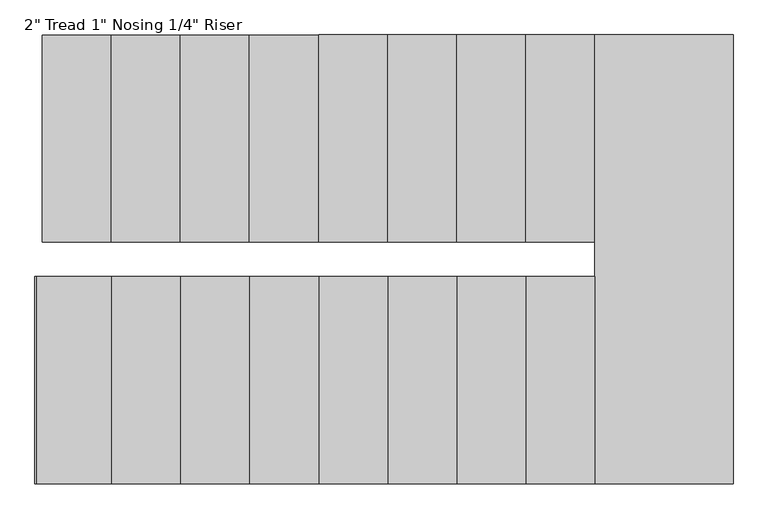
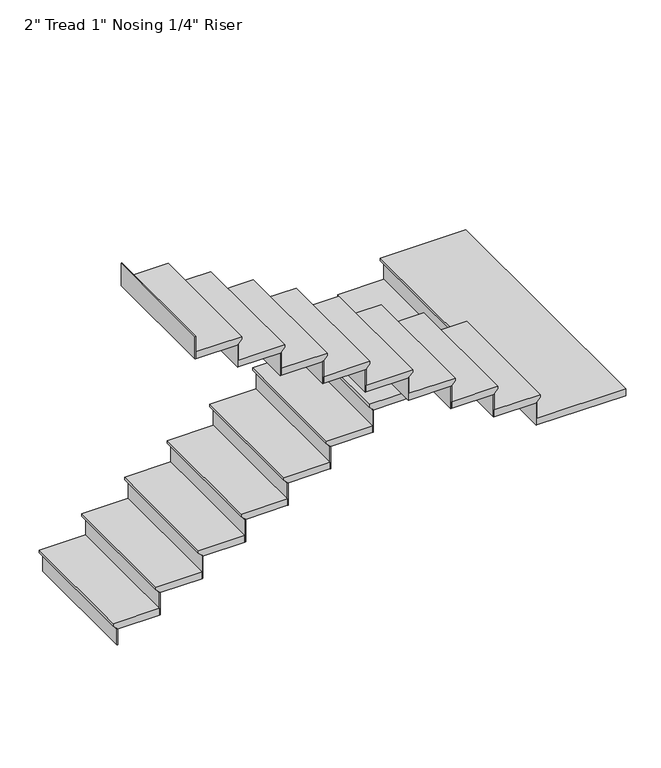
"""IFC4 building model written with IfcOpenShell, lengths in millimetres: stair flight geometry."""

from ifc_helpers import new_model, si_unit, origin, place, context, project, spatial, faceted_brep, source, transform, mapped, element, save


def stair_flight_ef7e9c63(model_context):
    return source(origin(), model_context, "Body", "Brep", [
        faceted_brep([(4699.0, 4356.1, 6246.2833333), (4699.0, 4356.1, 6265.3333333), (4699.0, 5270.5, 6265.3333333), (4699.0, 5270.5, 6246.2833333), (4724.4, 4356.1, 6220.8833333), (4724.4, 5270.5, 6220.8833333), (5029.2, 4356.1, 6265.3333333), (5029.2, 5270.5, 6265.3333333), (4724.4, 5270.5, 6214.5333333), (5029.2, 5270.5, 6214.5333333), (5029.2, 4356.1, 6214.5333333), (4724.4, 4356.1, 6214.5333333)], [[[0, 1, 2, 3]], [[4, 0, 3, 5]], [[2, 1, 6, 7]], [[8, 9, 10, 11]], [[2, 7, 9, 8, 5, 3]], [[8, 11, 4, 5]], [[6, 1, 0, 4, 11, 10]], [[7, 6, 10, 9]]]),
        faceted_brep([(4724.4, 4356.1, 6214.5333333), (4724.4, 4356.1, 6096.0), (4730.75, 4356.1, 6096.0), (4730.75, 4356.1, 6214.5333333), (4724.4, 5270.5, 6214.5333333), (4730.75, 5270.5, 6214.5333333), (4730.75, 5270.5, 6096.0), (4724.4, 5270.5, 6096.0)], [[[0, 1, 2, 3]], [[4, 5, 6, 7]], [[1, 0, 4, 7]], [[2, 1, 7, 6]], [[3, 2, 6, 5]], [[0, 3, 5, 4]]]),
        faceted_brep([(5029.2, 4356.1, 6383.8666667), (5029.2, 4356.1, 6214.5333333), (5035.55, 4356.1, 6214.5333333), (5035.55, 4356.1, 6383.8666667), (5029.2, 5270.5, 6383.8666667), (5035.55, 5270.5, 6383.8666667), (5035.55, 5270.5, 6214.5333333), (5029.2, 5270.5, 6214.5333333)], [[[0, 1, 2, 3]], [[4, 5, 6, 7]], [[1, 0, 4, 7]], [[2, 1, 7, 6]], [[3, 2, 6, 5]], [[0, 3, 5, 4]]]),
        faceted_brep([(5003.8, 5270.5, 6434.6666667), (5003.8, 4356.1, 6434.6666667), (5334.0, 4356.1, 6434.6666667), (5334.0, 5270.5, 6434.6666667), (5029.2, 5270.5, 6383.8666667), (5334.0, 5270.5, 6383.8666667), (5334.0, 4356.1, 6383.8666667), (5029.2, 4356.1, 6383.8666667), (5029.2, 5270.5, 6390.2166667), (5003.8, 5270.5, 6415.6166667), (5029.2, 4356.1, 6390.2166667), (5003.8, 4356.1, 6415.6166667)], [[[0, 1, 2, 3]], [[4, 5, 6, 7]], [[0, 3, 5, 4, 8, 9]], [[4, 7, 10, 8]], [[2, 1, 11, 10, 7, 6]], [[3, 2, 6, 5]], [[11, 1, 0, 9]], [[10, 11, 9, 8]]]),
        faceted_brep([(5334.0, 4356.1, 6553.2), (5334.0, 4356.1, 6383.8666667), (5340.35, 4356.1, 6383.8666667), (5340.35, 4356.1, 6553.2), (5334.0, 5270.5, 6553.2), (5340.35, 5270.5, 6553.2), (5340.35, 5270.5, 6383.8666667), (5334.0, 5270.5, 6383.8666667)], [[[0, 1, 2, 3]], [[4, 5, 6, 7]], [[1, 0, 4, 7]], [[2, 1, 7, 6]], [[3, 2, 6, 5]], [[0, 3, 5, 4]]]),
        faceted_brep([(5308.6, 5270.5, 6604.0), (5308.6, 4356.1, 6604.0), (5638.8, 4356.1, 6604.0), (5638.8, 5270.5, 6604.0), (5334.0, 5270.5, 6553.2), (5638.8, 5270.5, 6553.2), (5638.8, 4356.1, 6553.2), (5334.0, 4356.1, 6553.2), (5334.0, 5270.5, 6559.55), (5308.6, 5270.5, 6584.95), (5334.0, 4356.1, 6559.55), (5308.6, 4356.1, 6584.95)], [[[0, 1, 2, 3]], [[4, 5, 6, 7]], [[0, 3, 5, 4, 8, 9]], [[4, 7, 10, 8]], [[2, 1, 11, 10, 7, 6]], [[3, 2, 6, 5]], [[11, 1, 0, 9]], [[10, 11, 9, 8]]]),
        faceted_brep([(5638.8, 4356.1, 6722.5333333), (5638.8, 4356.1, 6553.2), (5645.15, 4356.1, 6553.2), (5645.15, 4356.1, 6722.5333333), (5638.8, 5270.5, 6722.5333333), (5645.15, 5270.5, 6722.5333333), (5645.15, 5270.5, 6553.2), (5638.8, 5270.5, 6553.2)], [[[0, 1, 2, 3]], [[4, 5, 6, 7]], [[1, 0, 4, 7]], [[2, 1, 7, 6]], [[3, 2, 6, 5]], [[0, 3, 5, 4]]]),
        faceted_brep([(5613.4, 5270.5, 6773.3333333), (5613.4, 4356.1, 6773.3333333), (5943.6, 4356.1, 6773.3333333), (5943.6, 5270.5, 6773.3333333), (5638.8, 5270.5, 6722.5333333), (5943.6, 5270.5, 6722.5333333), (5943.6, 4356.1, 6722.5333333), (5638.8, 4356.1, 6722.5333333), (5638.8, 5270.5, 6728.8833333), (5613.4, 5270.5, 6754.2833333), (5638.8, 4356.1, 6728.8833333), (5613.4, 4356.1, 6754.2833333)], [[[0, 1, 2, 3]], [[4, 5, 6, 7]], [[0, 3, 5, 4, 8, 9]], [[4, 7, 10, 8]], [[2, 1, 11, 10, 7, 6]], [[3, 2, 6, 5]], [[11, 1, 0, 9]], [[10, 11, 9, 8]]]),
        faceted_brep([(5943.6, 4356.1, 6891.8666667), (5943.6, 4356.1, 6722.5333333), (5949.95, 4356.1, 6722.5333333), (5949.95, 4356.1, 6891.8666667), (5943.6, 5270.5, 6891.8666667), (5949.95, 5270.5, 6891.8666667), (5949.95, 5270.5, 6722.5333333), (5943.6, 5270.5, 6722.5333333)], [[[0, 1, 2, 3]], [[4, 5, 6, 7]], [[1, 0, 4, 7]], [[2, 1, 7, 6]], [[3, 2, 6, 5]], [[0, 3, 5, 4]]]),
        faceted_brep([(5918.2, 5270.5, 6942.6666667), (5918.2, 4356.1, 6942.6666667), (6248.4, 4356.1, 6942.6666667), (6248.4, 5270.5, 6942.6666667), (5943.6, 5270.5, 6891.8666667), (6248.4, 5270.5, 6891.8666667), (6248.4, 4356.1, 6891.8666667), (5943.6, 4356.1, 6891.8666667), (5943.6, 5270.5, 6898.2166667), (5918.2, 5270.5, 6923.6166667), (5943.6, 4356.1, 6898.2166667), (5918.2, 4356.1, 6923.6166667)], [[[0, 1, 2, 3]], [[4, 5, 6, 7]], [[0, 3, 5, 4, 8, 9]], [[4, 7, 10, 8]], [[2, 1, 11, 10, 7, 6]], [[3, 2, 6, 5]], [[11, 1, 0, 9]], [[10, 11, 9, 8]]]),
        faceted_brep([(6248.4, 4356.1, 7061.2), (6248.4, 4356.1, 6891.8666667), (6254.75, 4356.1, 6891.8666667), (6254.75, 4356.1, 7061.2), (6248.4, 5270.5, 7061.2), (6254.75, 5270.5, 7061.2), (6254.75, 5270.5, 6891.8666667), (6248.4, 5270.5, 6891.8666667)], [[[0, 1, 2, 3]], [[4, 5, 6, 7]], [[1, 0, 4, 7]], [[2, 1, 7, 6]], [[3, 2, 6, 5]], [[0, 3, 5, 4]]]),
        faceted_brep([(6223.0, 5270.5, 7112.0), (6223.0, 4356.1, 7112.0), (6553.2, 4356.1, 7112.0), (6553.2, 5270.5, 7112.0), (6248.4, 5270.5, 7061.2), (6553.2, 5270.5, 7061.2), (6553.2, 4356.1, 7061.2), (6248.4, 4356.1, 7061.2), (6248.4, 5270.5, 7067.55), (6223.0, 5270.5, 7092.95), (6248.4, 4356.1, 7067.55), (6223.0, 4356.1, 7092.95)], [[[0, 1, 2, 3]], [[4, 5, 6, 7]], [[0, 3, 5, 4, 8, 9]], [[4, 7, 10, 8]], [[2, 1, 11, 10, 7, 6]], [[3, 2, 6, 5]], [[11, 1, 0, 9]], [[10, 11, 9, 8]]]),
        faceted_brep([(6553.2, 4356.1, 7230.5333333), (6553.2, 4356.1, 7061.2), (6559.55, 4356.1, 7061.2), (6559.55, 4356.1, 7230.5333333), (6553.2, 5270.5, 7230.5333333), (6559.55, 5270.5, 7230.5333333), (6559.55, 5270.5, 7061.2), (6553.2, 5270.5, 7061.2)], [[[0, 1, 2, 3]], [[4, 5, 6, 7]], [[1, 0, 4, 7]], [[2, 1, 7, 6]], [[3, 2, 6, 5]], [[0, 3, 5, 4]]]),
        faceted_brep([(6527.8, 5270.5, 7281.3333333), (6527.8, 4356.1, 7281.3333333), (6858.0, 4356.1, 7281.3333333), (6858.0, 5270.5, 7281.3333333), (6553.2, 5270.5, 7230.5333333), (6858.0, 5270.5, 7230.5333333), (6858.0, 4356.1, 7230.5333333), (6553.2, 4356.1, 7230.5333333), (6553.2, 5270.5, 7236.8833333), (6527.8, 5270.5, 7262.2833333), (6553.2, 4356.1, 7236.8833333), (6527.8, 4356.1, 7262.2833333)], [[[0, 1, 2, 3]], [[4, 5, 6, 7]], [[0, 3, 5, 4, 8, 9]], [[4, 7, 10, 8]], [[2, 1, 11, 10, 7, 6]], [[3, 2, 6, 5]], [[11, 1, 0, 9]], [[10, 11, 9, 8]]]),
        faceted_brep([(6858.0, 4356.1, 7399.8666667), (6858.0, 4356.1, 7230.5333333), (6864.35, 4356.1, 7230.5333333), (6864.35, 4356.1, 7399.8666667), (6858.0, 5270.5, 7399.8666667), (6864.35, 5270.5, 7399.8666667), (6864.35, 5270.5, 7230.5333333), (6858.0, 5270.5, 7230.5333333)], [[[0, 1, 2, 3]], [[4, 5, 6, 7]], [[1, 0, 4, 7]], [[2, 1, 7, 6]], [[3, 2, 6, 5]], [[0, 3, 5, 4]]]),
        faceted_brep([(6832.6, 5270.5, 7450.6666667), (6832.6, 4356.1, 7450.6666667), (7162.8, 4356.1, 7450.6666667), (7162.8, 5270.5, 7450.6666667), (6858.0, 5270.5, 7399.8666667), (7162.8, 5270.5, 7399.8666667), (7162.8, 4356.1, 7399.8666667), (6858.0, 4356.1, 7399.8666667), (6858.0, 5270.5, 7406.2166667), (6832.6, 5270.5, 7431.6166667), (6858.0, 4356.1, 7406.2166667), (6832.6, 4356.1, 7431.6166667)], [[[0, 1, 2, 3]], [[4, 5, 6, 7]], [[0, 3, 5, 4, 8, 9]], [[4, 7, 10, 8]], [[2, 1, 11, 10, 7, 6]], [[3, 2, 6, 5]], [[11, 1, 0, 9]], [[10, 11, 9, 8]]]),
        faceted_brep([(7162.8, 4356.1, 7569.2), (7162.8, 4356.1, 7399.8666667), (7169.15, 4356.1, 7399.8666667), (7169.15, 4356.1, 7569.2), (7162.8, 5270.5, 7569.2), (7169.15, 5270.5, 7569.2), (7169.15, 5270.5, 7399.8666667), (7162.8, 5270.5, 7399.8666667)], [[[0, 1, 2, 3]], [[4, 5, 6, 7]], [[1, 0, 4, 7]], [[2, 1, 7, 6]], [[3, 2, 6, 5]], [[0, 3, 5, 4]]]),
        faceted_brep([(7112.0, 3289.3, 7620.0), (7747.0, 3289.3, 7620.0), (7747.0, 5270.5, 7620.0), (7137.4, 5270.5, 7620.0), (7137.4, 4203.7, 7620.0), (7112.0, 4203.7, 7620.0), (7747.0, 3289.3, 7569.2), (7112.0, 3289.3, 7569.2), (7112.0, 4203.7, 7569.2), (7137.4, 4203.7, 7569.2), (7137.4, 4356.1, 7569.2), (7162.8, 4356.1, 7569.2), (7162.8, 5270.5, 7569.2), (7747.0, 5270.5, 7569.2), (7162.8, 5270.5, 7575.55), (7137.4, 5270.5, 7600.95), (7162.8, 4356.1, 7575.55), (7137.4, 4356.1, 7600.95)], [[[0, 1, 2, 3, 4, 5]], [[6, 7, 8, 9, 10, 11, 12, 13]], [[1, 0, 7, 6]], [[2, 1, 6, 13]], [[3, 2, 13, 12, 14, 15]], [[12, 11, 16, 14]], [[11, 10, 17, 16]], [[4, 3, 15, 17, 10, 9]], [[5, 4, 9, 8]], [[0, 5, 8, 7]], [[15, 14, 16, 17]]]),
        faceted_brep([(7112.0, 4203.7, 7738.5333333), (7112.0, 4203.7, 7569.2), (7105.65, 4203.7, 7569.2), (7105.65, 4203.7, 7738.5333333), (7112.0, 3289.3, 7738.5333333), (7105.65, 3289.3, 7738.5333333), (7105.65, 3289.3, 7569.2), (7112.0, 3289.3, 7569.2)], [[[0, 1, 2, 3]], [[4, 5, 6, 7]], [[1, 0, 4, 7]], [[2, 1, 7, 6]], [[3, 2, 6, 5]], [[0, 3, 5, 4]]]),
        faceted_brep([(7137.4, 3289.3, 7789.3333333), (7137.4, 4203.7, 7789.3333333), (6807.2, 4203.7, 7789.3333333), (6807.2, 3289.3, 7789.3333333), (7112.0, 3289.3, 7738.5333333), (6807.2, 3289.3, 7738.5333333), (6807.2, 4203.7, 7738.5333333), (7112.0, 4203.7, 7738.5333333), (7112.0, 3289.3, 7744.8833333), (7137.4, 3289.3, 7770.2833333), (7112.0, 4203.7, 7744.8833333), (7137.4, 4203.7, 7770.2833333)], [[[0, 1, 2, 3]], [[4, 5, 6, 7]], [[0, 3, 5, 4, 8, 9]], [[4, 7, 10, 8]], [[2, 1, 11, 10, 7, 6]], [[3, 2, 6, 5]], [[11, 1, 0, 9]], [[10, 11, 9, 8]]]),
        faceted_brep([(6807.2, 4203.7, 7907.8666667), (6807.2, 4203.7, 7738.5333333), (6800.85, 4203.7, 7738.5333333), (6800.85, 4203.7, 7907.8666667), (6807.2, 3289.3, 7907.8666667), (6800.85, 3289.3, 7907.8666667), (6800.85, 3289.3, 7738.5333333), (6807.2, 3289.3, 7738.5333333)], [[[0, 1, 2, 3]], [[4, 5, 6, 7]], [[1, 0, 4, 7]], [[2, 1, 7, 6]], [[3, 2, 6, 5]], [[0, 3, 5, 4]]]),
        faceted_brep([(6832.6, 3289.3, 7958.6666667), (6832.6, 4203.7, 7958.6666667), (6502.4, 4203.7, 7958.6666667), (6502.4, 3289.3, 7958.6666667), (6807.2, 3289.3, 7907.8666667), (6502.4, 3289.3, 7907.8666667), (6502.4, 4203.7, 7907.8666667), (6807.2, 4203.7, 7907.8666667), (6807.2, 3289.3, 7914.2166667), (6832.6, 3289.3, 7939.6166667), (6807.2, 4203.7, 7914.2166667), (6832.6, 4203.7, 7939.6166667)], [[[0, 1, 2, 3]], [[4, 5, 6, 7]], [[0, 3, 5, 4, 8, 9]], [[4, 7, 10, 8]], [[2, 1, 11, 10, 7, 6]], [[3, 2, 6, 5]], [[11, 1, 0, 9]], [[10, 11, 9, 8]]]),
        faceted_brep([(6502.4, 4203.7, 8077.2), (6502.4, 4203.7, 7907.8666667), (6496.05, 4203.7, 7907.8666667), (6496.05, 4203.7, 8077.2), (6502.4, 3289.3, 8077.2), (6496.05, 3289.3, 8077.2), (6496.05, 3289.3, 7907.8666667), (6502.4, 3289.3, 7907.8666667)], [[[0, 1, 2, 3]], [[4, 5, 6, 7]], [[1, 0, 4, 7]], [[2, 1, 7, 6]], [[3, 2, 6, 5]], [[0, 3, 5, 4]]]),
        faceted_brep([(6527.8, 3289.3, 8128.0), (6527.8, 4203.7, 8128.0), (6197.6, 4203.7, 8128.0), (6197.6, 3289.3, 8128.0), (6502.4, 3289.3, 8077.2), (6197.6, 3289.3, 8077.2), (6197.6, 4203.7, 8077.2), (6502.4, 4203.7, 8077.2), (6502.4, 3289.3, 8083.55), (6527.8, 3289.3, 8108.95), (6502.4, 4203.7, 8083.55), (6527.8, 4203.7, 8108.95)], [[[0, 1, 2, 3]], [[4, 5, 6, 7]], [[0, 3, 5, 4, 8, 9]], [[4, 7, 10, 8]], [[2, 1, 11, 10, 7, 6]], [[3, 2, 6, 5]], [[11, 1, 0, 9]], [[10, 11, 9, 8]]]),
        faceted_brep([(6197.6, 4203.7, 8246.5333333), (6197.6, 4203.7, 8077.2), (6191.25, 4203.7, 8077.2), (6191.25, 4203.7, 8246.5333333), (6197.6, 3289.3, 8246.5333333), (6191.25, 3289.3, 8246.5333333), (6191.25, 3289.3, 8077.2), (6197.6, 3289.3, 8077.2)], [[[0, 1, 2, 3]], [[4, 5, 6, 7]], [[1, 0, 4, 7]], [[2, 1, 7, 6]], [[3, 2, 6, 5]], [[0, 3, 5, 4]]]),
        faceted_brep([(6223.0, 3289.3, 8297.3333333), (6223.0, 4203.7, 8297.3333333), (5892.8, 4203.7, 8297.3333333), (5892.8, 3289.3, 8297.3333333), (6197.6, 3289.3, 8246.5333333), (5892.8, 3289.3, 8246.5333333), (5892.8, 4203.7, 8246.5333333), (6197.6, 4203.7, 8246.5333333), (6197.6, 3289.3, 8252.8833333), (6223.0, 3289.3, 8278.2833333), (6197.6, 4203.7, 8252.8833333), (6223.0, 4203.7, 8278.2833333)], [[[0, 1, 2, 3]], [[4, 5, 6, 7]], [[0, 3, 5, 4, 8, 9]], [[4, 7, 10, 8]], [[2, 1, 11, 10, 7, 6]], [[3, 2, 6, 5]], [[11, 1, 0, 9]], [[10, 11, 9, 8]]]),
        faceted_brep([(5892.8, 4203.7, 8415.8666667), (5892.8, 4203.7, 8246.5333333), (5886.45, 4203.7, 8246.5333333), (5886.45, 4203.7, 8415.8666667), (5892.8, 3289.3, 8415.8666667), (5886.45, 3289.3, 8415.8666667), (5886.45, 3289.3, 8246.5333333), (5892.8, 3289.3, 8246.5333333)], [[[0, 1, 2, 3]], [[4, 5, 6, 7]], [[1, 0, 4, 7]], [[2, 1, 7, 6]], [[3, 2, 6, 5]], [[0, 3, 5, 4]]]),
        faceted_brep([(5918.2, 3289.3, 8466.6666667), (5918.2, 4203.7, 8466.6666667), (5588.0, 4203.7, 8466.6666667), (5588.0, 3289.3, 8466.6666667), (5892.8, 3289.3, 8415.8666667), (5588.0, 3289.3, 8415.8666667), (5588.0, 4203.7, 8415.8666667), (5892.8, 4203.7, 8415.8666667), (5892.8, 3289.3, 8422.2166667), (5918.2, 3289.3, 8447.6166667), (5892.8, 4203.7, 8422.2166667), (5918.2, 4203.7, 8447.6166667)], [[[0, 1, 2, 3]], [[4, 5, 6, 7]], [[0, 3, 5, 4, 8, 9]], [[4, 7, 10, 8]], [[2, 1, 11, 10, 7, 6]], [[3, 2, 6, 5]], [[11, 1, 0, 9]], [[10, 11, 9, 8]]]),
        faceted_brep([(5588.0, 4203.7, 8585.2), (5588.0, 4203.7, 8415.8666667), (5581.65, 4203.7, 8415.8666667), (5581.65, 4203.7, 8585.2), (5588.0, 3289.3, 8585.2), (5581.65, 3289.3, 8585.2), (5581.65, 3289.3, 8415.8666667), (5588.0, 3289.3, 8415.8666667)], [[[0, 1, 2, 3]], [[4, 5, 6, 7]], [[1, 0, 4, 7]], [[2, 1, 7, 6]], [[3, 2, 6, 5]], [[0, 3, 5, 4]]]),
        faceted_brep([(5613.4, 3289.3, 8636.0), (5613.4, 4203.7, 8636.0), (5283.2, 4203.7, 8636.0), (5283.2, 3289.3, 8636.0), (5588.0, 3289.3, 8585.2), (5283.2, 3289.3, 8585.2), (5283.2, 4203.7, 8585.2), (5588.0, 4203.7, 8585.2), (5588.0, 3289.3, 8591.55), (5613.4, 3289.3, 8616.95), (5588.0, 4203.7, 8591.55), (5613.4, 4203.7, 8616.95)], [[[0, 1, 2, 3]], [[4, 5, 6, 7]], [[0, 3, 5, 4, 8, 9]], [[4, 7, 10, 8]], [[2, 1, 11, 10, 7, 6]], [[3, 2, 6, 5]], [[11, 1, 0, 9]], [[10, 11, 9, 8]]]),
        faceted_brep([(5283.2, 4203.7, 8754.5333333), (5283.2, 4203.7, 8585.2), (5276.85, 4203.7, 8585.2), (5276.85, 4203.7, 8754.5333333), (5283.2, 3289.3, 8754.5333333), (5276.85, 3289.3, 8754.5333333), (5276.85, 3289.3, 8585.2), (5283.2, 3289.3, 8585.2)], [[[0, 1, 2, 3]], [[4, 5, 6, 7]], [[1, 0, 4, 7]], [[2, 1, 7, 6]], [[3, 2, 6, 5]], [[0, 3, 5, 4]]]),
        faceted_brep([(5308.6, 3289.3, 8805.3333333), (5308.6, 4203.7, 8805.3333333), (4978.4, 4203.7, 8805.3333333), (4978.4, 3289.3, 8805.3333333), (5283.2, 3289.3, 8754.5333333), (4978.4, 3289.3, 8754.5333333), (4978.4, 4203.7, 8754.5333333), (5283.2, 4203.7, 8754.5333333), (5283.2, 3289.3, 8760.8833333), (5308.6, 3289.3, 8786.2833333), (5283.2, 4203.7, 8760.8833333), (5308.6, 4203.7, 8786.2833333)], [[[0, 1, 2, 3]], [[4, 5, 6, 7]], [[0, 3, 5, 4, 8, 9]], [[4, 7, 10, 8]], [[2, 1, 11, 10, 7, 6]], [[3, 2, 6, 5]], [[11, 1, 0, 9]], [[10, 11, 9, 8]]]),
        faceted_brep([(4978.4, 4203.7, 8923.8666667), (4978.4, 4203.7, 8754.5333333), (4972.05, 4203.7, 8754.5333333), (4972.05, 4203.7, 8923.8666667), (4978.4, 3289.3, 8923.8666667), (4972.05, 3289.3, 8923.8666667), (4972.05, 3289.3, 8754.5333333), (4978.4, 3289.3, 8754.5333333)], [[[0, 1, 2, 3]], [[4, 5, 6, 7]], [[1, 0, 4, 7]], [[2, 1, 7, 6]], [[3, 2, 6, 5]], [[0, 3, 5, 4]]]),
        faceted_brep([(4673.6, 4203.7, 9093.2), (4673.6, 4203.7, 8923.8666667), (4667.25, 4203.7, 8923.8666667), (4667.25, 4203.7, 9093.2), (4673.6, 3289.3, 9093.2), (4667.25, 3289.3, 9093.2), (4667.25, 3289.3, 8923.8666667), (4673.6, 3289.3, 8923.8666667)], [[[0, 1, 2, 3]], [[4, 5, 6, 7]], [[1, 0, 4, 7]], [[2, 1, 7, 6]], [[3, 2, 6, 5]], [[0, 3, 5, 4]]]),
        faceted_brep([(5003.8, 3289.3, 8974.6666667), (5003.8, 4203.7, 8974.6666667), (4673.6, 4203.7, 8974.6666667), (4673.6, 3289.3, 8974.6666667), (4978.4, 3289.3, 8923.8666667), (4673.6, 3289.3, 8923.8666667), (4673.6, 4203.7, 8923.8666667), (4978.4, 4203.7, 8923.8666667), (4978.4, 3289.3, 8930.2166667), (5003.8, 3289.3, 8955.6166667), (4978.4, 4203.7, 8930.2166667), (5003.8, 4203.7, 8955.6166667)], [[[0, 1, 2, 3]], [[4, 5, 6, 7]], [[0, 3, 5, 4, 8, 9]], [[4, 7, 10, 8]], [[2, 1, 11, 10, 7, 6]], [[3, 2, 6, 5]], [[11, 1, 0, 9]], [[10, 11, 9, 8]]]),
    ])


if __name__ == "__main__":
    model = new_model("IFC4")
    model_context = context("Model", 3, world=origin())
    ifc_project = project(units=[si_unit("LENGTHUNIT", "METRE", prefix="MILLI")], contexts=[model_context])
    site = spatial("IfcSite", under=ifc_project)
    building = spatial("IfcBuilding", under=site)
    placement = place(None, origin())
    stair_flight_shape = stair_flight_ef7e9c63(model_context)
    element("IfcStairFlight", 1, ObjectType="2\" Tread 1\" Nosing 1/4\" Riser", at=placement, inside=building, context=model_context, shape_type="MappedRepresentation", body=[
        mapped(stair_flight_shape, transform((0.0, 0.0, 0.0), x_axis=(1.0, 0.0, 0.0), y_axis=(0.0, 1.0, 0.0), z_axis=(0.0, 0.0, 1.0))),
    ])
    save(model, "model.ifc")
